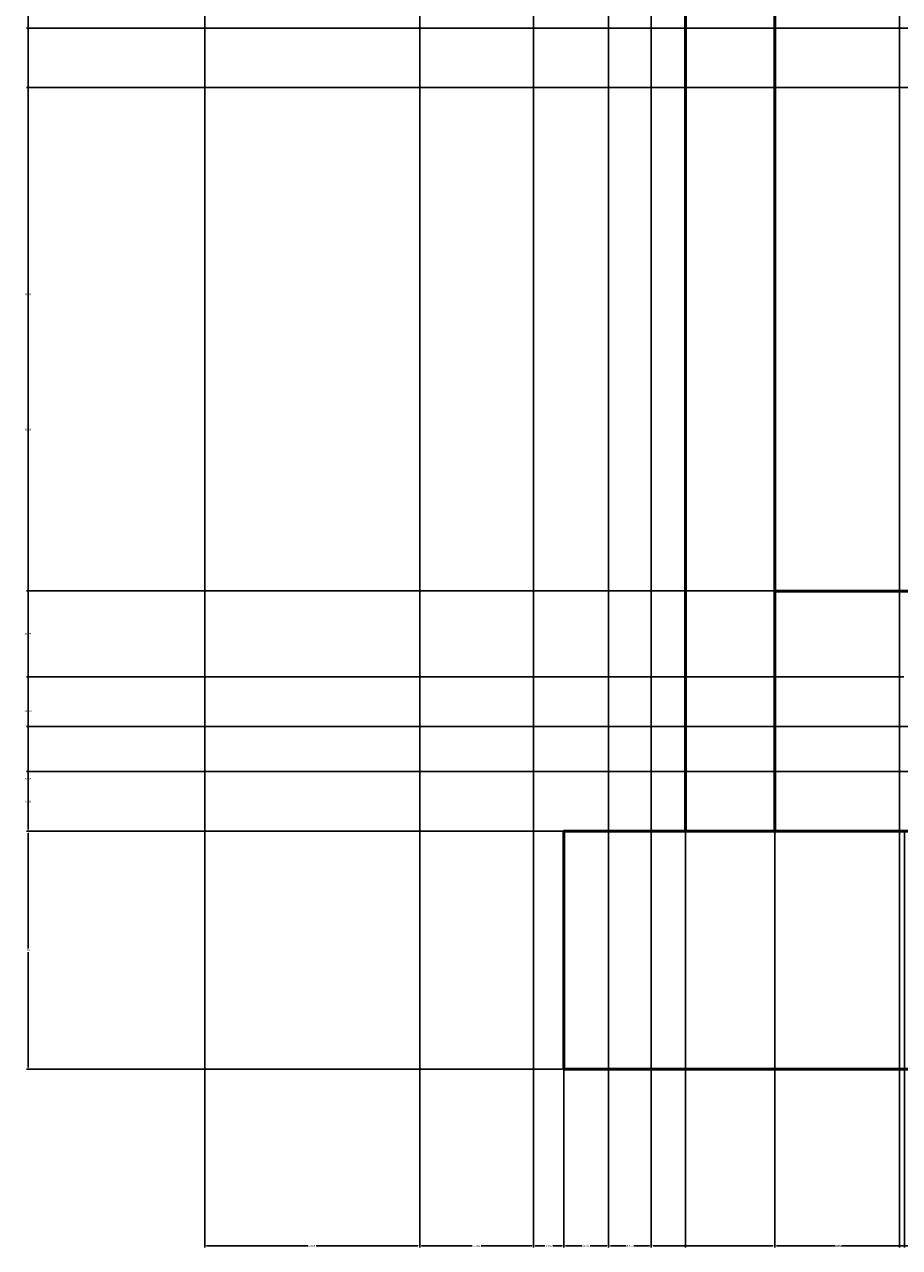
# Model space of a CAD drawing. Units: inches. Extents: x 27 to 409, y -26 to 294.
# Tile 1 of 7: x 27 to 116, y -26 to 97. Entities that reach past the tile are written whole.
import ezdxf

# ---------------------------------------------------------------- set-up
doc = ezdxf.new("R2010")
doc.units = ezdxf.units.IN
doc.header["$MEASUREMENT"] = 0
doc.layers.add('A-ANNO-DIMS', color=2, linetype='Continuous', lineweight=18)
doc.layers.add('A-WALL', color=7, linetype='Continuous', lineweight=50)
doc.styles.get("Standard").update_dxf_attribs({"font": 'arial.ttf'})
doc.dimstyles.get("Standard").update_dxf_attribs({"dimtxt": 0.18, "dimasz": 0.18, "dimexe": 0.18, "dimexo": 0.0625, "dimgap": 0.09, "dimtad": 0, "dimtih": 1, "dimtoh": 1, "dimdec": 4, "dimzin": 0, "dimdsep": 46, "dimtxsty": 'Standard', "dimcen": 0.09, "dimadec": 0, "dimazin": 0, "dimtfac": 1, "dimtdec": 4, "dimtofl": 0, "dimtmove": 0, "dimatfit": 3, "dimfxl": 1, "dimtolj": 1, "dimtzin": 0, "dimarcsym": 0})

# ---------------------------------------------------------------- blocks, each defined once
blk = doc.blocks.new('*D8')
at = {"layer": 'A-ANNO-DIMS', "color": 0, "lineweight": -2, "transparency": 16777216}
for p, q in [((67.27, 209.05), (67.27, -26.5)), ((45.58, 99.43), (45.58, -26.5)), ((45.76, -26.32), (56.03, -26.32)), ((67.09, -26.32), (56.82, -26.32))]:
    blk.add_line(p, q, dxfattribs=at)
at = {"layer": 'A-ANNO-DIMS', "color": 0, "transparency": 16777216}
for points in [[(45.76, -26.29), (45.76, -26.35), (45.58, -26.32)], [(67.09, -26.29), (67.09, -26.35), (67.27, -26.32)]]:
    blk.add_solid(points, dxfattribs=at)
at = {"layer": 'Defpoints', "color": 0, "transparency": 16777216}
for p in [(67.27, 209.11), (45.58, 99.5), (67.27, -26.32)]:
    blk.add_point(p, dxfattribs=at)
at = {"layer": 'A-ANNO-DIMS', "color": 0, "transparency": 16777216, "insert": (56.42, -26.32), "char_height": 0.18, "attachment_point": 5}
blk.add_mtext('\\A1;21.69', dxfattribs=at)
blk = doc.blocks.new('*D9')
at = {"layer": 'A-ANNO-DIMS', "color": 0, "lineweight": -2, "transparency": 16777216}
for p, q in [((78.75, 231.7), (78.75, -26.5)), ((67.27, 209.05), (67.27, -26.5)), ((67.45, -26.32), (72.55, -26.32)), ((78.57, -26.32), (73.46, -26.32))]:
    blk.add_line(p, q, dxfattribs=at)
at = {"layer": 'A-ANNO-DIMS', "color": 0, "transparency": 16777216}
for points in [[(67.45, -26.29), (67.45, -26.35), (67.27, -26.32)], [(78.57, -26.29), (78.57, -26.35), (78.75, -26.32)]]:
    blk.add_solid(points, dxfattribs=at)
at = {"layer": 'Defpoints', "color": 0, "transparency": 16777216}
for p in [(78.75, 231.76), (67.27, 209.11), (78.75, -26.32)]:
    blk.add_point(p, dxfattribs=at)
at = {"layer": 'A-ANNO-DIMS', "color": 0, "transparency": 16777216, "insert": (73.01, -26.32), "char_height": 0.18, "attachment_point": 5}
blk.add_mtext('\\A1;11.482', dxfattribs=at)
blk = doc.blocks.new('*D10')
at = {"layer": 'A-ANNO-DIMS', "color": 0, "lineweight": -2, "transparency": 16777216}
for p, q in [((78.75, 231.7), (78.75, -26.5)), ((81.81, -8.58), (81.81, -26.5)), ((78.93, -26.32), (79.89, -26.32)), ((81.63, -26.32), (80.68, -26.32))]:
    blk.add_line(p, q, dxfattribs=at)
at = {"layer": 'A-ANNO-DIMS', "color": 0, "transparency": 16777216}
for points in [[(78.93, -26.29), (78.93, -26.35), (78.75, -26.32)], [(81.63, -26.29), (81.63, -26.35), (81.81, -26.32)]]:
    blk.add_solid(points, dxfattribs=at)
at = {"layer": 'Defpoints', "color": 0, "transparency": 16777216}
for p in [(78.75, 231.76), (81.81, -8.52), (81.81, -26.32)]:
    blk.add_point(p, dxfattribs=at)
at = {"layer": 'A-ANNO-DIMS', "color": 0, "transparency": 16777216, "insert": (80.28, -26.32), "char_height": 0.18, "attachment_point": 5}
blk.add_mtext('\\A1;3.064', dxfattribs=at)
blk = doc.blocks.new('*D11')
at = {"layer": 'A-ANNO-DIMS', "color": 0, "lineweight": -2, "transparency": 16777216}
for p, q in [((86.32, 163.84), (86.32, -26.5)), ((81.81, -8.58), (81.81, -26.5)), ((81.99, -26.32), (83.67, -26.32)), ((86.14, -26.32), (84.46, -26.32))]:
    blk.add_line(p, q, dxfattribs=at)
at = {"layer": 'A-ANNO-DIMS', "color": 0, "transparency": 16777216}
for points in [[(81.99, -26.29), (81.99, -26.35), (81.81, -26.32)], [(86.14, -26.29), (86.14, -26.35), (86.32, -26.32)]]:
    blk.add_solid(points, dxfattribs=at)
at = {"layer": 'Defpoints', "color": 0, "transparency": 16777216}
for p in [(86.32, 163.9), (81.81, -8.52), (86.32, -26.32)]:
    blk.add_point(p, dxfattribs=at)
at = {"layer": 'A-ANNO-DIMS', "color": 0, "transparency": 16777216, "insert": (84.07, -26.32), "char_height": 0.18, "attachment_point": 5}
blk.add_mtext('\\A1;4.503', dxfattribs=at)
blk = doc.blocks.new('*D12')
at = {"layer": 'A-ANNO-DIMS', "color": 0, "lineweight": -2, "transparency": 16777216}
for p, q in [((90.63, 195.36), (90.63, -26.5)), ((86.32, 163.84), (86.32, -26.5)), ((86.5, -26.32), (88.09, -26.32)), ((90.45, -26.32), (88.85, -26.32))]:
    blk.add_line(p, q, dxfattribs=at)
at = {"layer": 'A-ANNO-DIMS', "color": 0, "transparency": 16777216}
for points in [[(86.5, -26.29), (86.5, -26.35), (86.32, -26.32)], [(90.45, -26.29), (90.45, -26.35), (90.63, -26.32)]]:
    blk.add_solid(points, dxfattribs=at)
at = {"layer": 'Defpoints', "color": 0, "transparency": 16777216}
for p in [(90.63, 195.42), (86.32, 163.9), (90.63, -26.32)]:
    blk.add_point(p, dxfattribs=at)
at = {"layer": 'A-ANNO-DIMS', "color": 0, "transparency": 16777216, "insert": (88.47, -26.32), "char_height": 0.18, "attachment_point": 5}
blk.add_mtext('\\A1;4.311', dxfattribs=at)
blk = doc.blocks.new('*D13')
at = {"layer": 'A-ANNO-DIMS', "color": 0, "lineweight": -2, "transparency": 16777216}
for p, q in [((90.63, 195.36), (90.63, -26.5)), ((103.08, 162.87), (103.08, -26.5)), ((90.81, -26.32), (96.4, -26.32)), ((102.9, -26.32), (97.31, -26.32))]:
    blk.add_line(p, q, dxfattribs=at)
at = {"layer": 'A-ANNO-DIMS', "color": 0, "transparency": 16777216}
for points in [[(90.81, -26.29), (90.81, -26.35), (90.63, -26.32)], [(102.9, -26.29), (102.9, -26.35), (103.08, -26.32)]]:
    blk.add_solid(points, dxfattribs=at)
at = {"layer": 'Defpoints', "color": 0, "transparency": 16777216}
for p in [(90.63, 195.42), (103.08, 162.94), (103.08, -26.32)]:
    blk.add_point(p, dxfattribs=at)
at = {"layer": 'A-ANNO-DIMS', "color": 0, "transparency": 16777216, "insert": (96.85, -26.32), "char_height": 0.18, "attachment_point": 5}
blk.add_mtext('\\A1;12.447', dxfattribs=at)
blk = doc.blocks.new('*D14')
at = {"layer": 'A-ANNO-DIMS', "color": 0, "lineweight": -2, "transparency": 16777216}
for p, q in [((103.08, 162.87), (103.08, -26.5)), ((115.67, 115.93), (115.67, -26.5)), ((103.26, -26.32), (108.93, -26.32)), ((115.49, -26.32), (109.81, -26.32))]:
    blk.add_line(p, q, dxfattribs=at)
at = {"layer": 'A-ANNO-DIMS', "color": 0, "transparency": 16777216}
for points in [[(103.26, -26.29), (103.26, -26.35), (103.08, -26.32)], [(115.49, -26.29), (115.49, -26.35), (115.67, -26.32)]]:
    blk.add_solid(points, dxfattribs=at)
at = {"layer": 'Defpoints', "color": 0, "transparency": 16777216}
for p in [(103.08, 162.94), (115.67, 116), (115.67, -26.32)]:
    blk.add_point(p, dxfattribs=at)
at = {"layer": 'A-ANNO-DIMS', "color": 0, "transparency": 16777216, "insert": (109.37, -26.32), "char_height": 0.18, "attachment_point": 5}
blk.add_mtext('\\A1;12.591', dxfattribs=at)
blk = doc.blocks.new('*D15')
at = {"layer": 'A-ANNO-DIMS', "color": 0, "lineweight": -2, "transparency": 16777216}
for p, q in [((152.83, 275.59), (152.83, -26.5)), ((115.67, 115.93), (115.67, -26.5)), ((115.85, -26.32), (133.86, -26.32)), ((152.65, -26.32), (134.64, -26.32))]:
    blk.add_line(p, q, dxfattribs=at)
at = {"layer": 'A-ANNO-DIMS', "color": 0, "transparency": 16777216}
for points in [[(115.85, -26.29), (115.85, -26.35), (115.67, -26.32)], [(152.65, -26.29), (152.65, -26.35), (152.83, -26.32)]]:
    blk.add_solid(points, dxfattribs=at)
at = {"layer": 'Defpoints', "color": 0, "transparency": 16777216}
for p in [(152.83, 275.65), (115.67, 116), (152.83, -26.32)]:
    blk.add_point(p, dxfattribs=at)
at = {"layer": 'A-ANNO-DIMS', "color": 0, "transparency": 16777216, "insert": (134.25, -26.32), "char_height": 0.18, "attachment_point": 5}
blk.add_mtext('\\A1;37.17', dxfattribs=at)
blk = doc.blocks.new('*D26')
at = {"layer": 'A-ANNO-DIMS', "color": 0, "lineweight": -2, "transparency": 16777216}
for p, q in [((81.75, 15.48), (27.6, 15.48)), ((27.78, 15.3), (27.78, 3.66)), ((27.78, -8.34), (27.78, 3.3)), ((81.75, -8.52), (27.6, -8.52))]:
    blk.add_line(p, q, dxfattribs=at)
at = {"layer": 'A-ANNO-DIMS', "color": 0, "transparency": 16777216}
for points in [[(27.75, 15.3), (27.81, 15.3), (27.78, 15.48)], [(27.75, -8.34), (27.81, -8.34), (27.78, -8.52)]]:
    blk.add_solid(points, dxfattribs=at)
at = {"layer": 'Defpoints', "color": 0, "transparency": 16777216}
for p in [(27.78, 15.48), (81.81, 15.48), (81.81, -8.52)]:
    blk.add_point(p, dxfattribs=at)
at = {"layer": 'A-ANNO-DIMS', "color": 0, "transparency": 16777216, "insert": (27.78, 3.48), "char_height": 0.18, "attachment_point": 5}
blk.add_mtext('\\A1;24', dxfattribs=at)
blk = doc.blocks.new('*D27')
at = {"layer": 'A-ANNO-DIMS', "color": 0, "lineweight": -2, "transparency": 16777216}
for p, q in [((115.6, 39.71), (27.6, 39.71)), ((27.78, 39.53), (27.78, 27.78)), ((27.78, 15.66), (27.78, 27.42)), ((81.75, 15.48), (27.6, 15.48))]:
    blk.add_line(p, q, dxfattribs=at)
at = {"layer": 'A-ANNO-DIMS', "color": 0, "transparency": 16777216}
for points in [[(27.75, 39.53), (27.81, 39.53), (27.78, 39.71)], [(27.75, 15.66), (27.81, 15.66), (27.78, 15.48)]]:
    blk.add_solid(points, dxfattribs=at)
at = {"layer": 'Defpoints', "color": 0, "transparency": 16777216}
for p in [(27.78, 39.71), (115.67, 39.71), (81.81, 15.48)]:
    blk.add_point(p, dxfattribs=at)
at = {"layer": 'A-ANNO-DIMS', "color": 0, "transparency": 16777216, "insert": (27.78, 27.6), "char_height": 0.18, "attachment_point": 5}
blk.add_mtext('\\A1;24.227', dxfattribs=at)
blk = doc.blocks.new('*D28')
at = {"layer": 'A-ANNO-DIMS', "color": 0, "lineweight": -2, "transparency": 16777216}
for p, q in [((45.51, 99.5), (27.6, 99.5)), ((27.78, 99.32), (27.78, 69.78)), ((27.78, 39.89), (27.78, 69.42)), ((115.6, 39.71), (27.6, 39.71))]:
    blk.add_line(p, q, dxfattribs=at)
at = {"layer": 'A-ANNO-DIMS', "color": 0, "transparency": 16777216}
for points in [[(27.75, 99.32), (27.81, 99.32), (27.78, 99.5)], [(27.75, 39.89), (27.81, 39.89), (27.78, 39.71)]]:
    blk.add_solid(points, dxfattribs=at)
at = {"layer": 'Defpoints', "color": 0, "transparency": 16777216}
for p in [(27.78, 99.5), (45.58, 99.5), (115.67, 39.71)]:
    blk.add_point(p, dxfattribs=at)
at = {"layer": 'A-ANNO-DIMS', "color": 0, "transparency": 16777216, "insert": (27.78, 69.6), "char_height": 0.18, "attachment_point": 5}
blk.add_mtext('\\A1;59.79', dxfattribs=at)
blk = doc.blocks.new('*D69')
at = {"layer": 'A-ANNO-DIMS', "color": 0, "lineweight": -2, "transparency": 16777216}
for p, q in [((200.04, 21.5), (27.6, 21.5)), ((27.78, 21.32), (27.78, 18.67)), ((27.78, 15.66), (27.78, 18.31)), ((190.01, 15.48), (27.6, 15.48))]:
    blk.add_line(p, q, dxfattribs=at)
at = {"layer": 'A-ANNO-DIMS', "color": 0, "transparency": 16777216}
for points in [[(27.75, 21.32), (27.81, 21.32), (27.78, 21.5)], [(27.75, 15.66), (27.81, 15.66), (27.78, 15.48)]]:
    blk.add_solid(points, dxfattribs=at)
at = {"layer": 'Defpoints', "color": 0, "transparency": 16777216}
for p in [(27.78, 21.5), (200.1, 21.5), (190.08, 15.48)]:
    blk.add_point(p, dxfattribs=at)
at = {"layer": 'A-ANNO-DIMS', "color": 0, "transparency": 16777216, "insert": (27.78, 18.49), "char_height": 0.18, "attachment_point": 5}
blk.add_mtext('\\A1;6.013', dxfattribs=at)
blk = doc.blocks.new('*D70')
at = {"layer": 'A-ANNO-DIMS', "color": 0, "lineweight": -2, "transparency": 16777216}
for p, q in [((200.04, 90.47), (27.6, 90.47)), ((27.78, 90.29), (27.78, 56.17)), ((27.78, 21.68), (27.78, 55.8)), ((200.04, 21.5), (27.6, 21.5))]:
    blk.add_line(p, q, dxfattribs=at)
at = {"layer": 'A-ANNO-DIMS', "color": 0, "transparency": 16777216}
for points in [[(27.75, 90.29), (27.81, 90.29), (27.78, 90.47)], [(27.75, 21.68), (27.81, 21.68), (27.78, 21.5)]]:
    blk.add_solid(points, dxfattribs=at)
at = {"layer": 'Defpoints', "color": 0, "transparency": 16777216}
for p in [(27.78, 90.47), (200.1, 90.47), (200.1, 21.5)]:
    blk.add_point(p, dxfattribs=at)
at = {"layer": 'A-ANNO-DIMS', "color": 0, "transparency": 16777216, "insert": (27.78, 55.98), "char_height": 0.18, "attachment_point": 5}
blk.add_mtext('\\A1;68.98', dxfattribs=at)
blk = doc.blocks.new('*D71')
at = {"layer": 'A-ANNO-DIMS', "color": 0, "lineweight": -2, "transparency": 16777216}
for p, q in [((196.04, 96.47), (27.6, 96.47)), ((27.78, 96.29), (27.78, 93.65)), ((27.78, 90.65), (27.78, 93.29)), ((200.04, 90.47), (27.6, 90.47))]:
    blk.add_line(p, q, dxfattribs=at)
at = {"layer": 'A-ANNO-DIMS', "color": 0, "transparency": 16777216}
for points in [[(27.75, 96.29), (27.81, 96.29), (27.78, 96.47)], [(27.75, 90.65), (27.81, 90.65), (27.78, 90.47)]]:
    blk.add_solid(points, dxfattribs=at)
at = {"layer": 'Defpoints', "color": 0, "transparency": 16777216}
for p in [(27.78, 96.47), (196.1, 96.47), (200.1, 90.47)]:
    blk.add_point(p, dxfattribs=at)
at = {"layer": 'A-ANNO-DIMS', "color": 0, "transparency": 16777216, "insert": (27.78, 93.47), "char_height": 0.18, "attachment_point": 5}
blk.add_mtext('\\A1;6', dxfattribs=at)
blk = doc.blocks.new('*D72')
at = {"layer": 'A-ANNO-DIMS', "color": 0, "lineweight": -2, "transparency": 16777216}
for p, q in [((190.01, 99.5), (27.6, 99.5)), ((27.78, 99.32), (27.78, 98.17)), ((27.78, 96.65), (27.78, 97.8)), ((196.04, 96.47), (27.6, 96.47))]:
    blk.add_line(p, q, dxfattribs=at)
at = {"layer": 'A-ANNO-DIMS', "color": 0, "transparency": 16777216}
for points in [[(27.75, 99.32), (27.81, 99.32), (27.78, 99.5)], [(27.75, 96.65), (27.81, 96.65), (27.78, 96.47)]]:
    blk.add_solid(points, dxfattribs=at)
at = {"layer": 'Defpoints', "color": 0, "transparency": 16777216}
for p in [(27.78, 99.5), (190.08, 99.5), (196.1, 96.47)]:
    blk.add_point(p, dxfattribs=at)
at = {"layer": 'A-ANNO-DIMS', "color": 0, "transparency": 16777216, "insert": (27.78, 97.98), "char_height": 0.18, "attachment_point": 5}
blk.add_mtext('\\A1;3.023', dxfattribs=at)
blk = doc.blocks.new('*D90')
at = {"layer": 'A-ANNO-DIMS', "color": 0, "lineweight": -2, "transparency": 16777216}
for p, q in [((94.08, 15.42), (94.08, -26.5)), ((103.08, 15.42), (103.08, -26.5)), ((94.26, -26.32), (98.43, -26.32)), ((102.9, -26.32), (98.72, -26.32))]:
    blk.add_line(p, q, dxfattribs=at)
at = {"layer": 'A-ANNO-DIMS', "color": 0, "transparency": 16777216}
for points in [[(94.26, -26.29), (94.26, -26.35), (94.08, -26.32)], [(102.9, -26.29), (102.9, -26.35), (103.08, -26.32)]]:
    blk.add_solid(points, dxfattribs=at)
at = {"layer": 'Defpoints', "color": 0, "transparency": 16777216}
for p in [(94.08, 15.48), (103.08, 15.48), (103.08, -26.32)]:
    blk.add_point(p, dxfattribs=at)
at = {"layer": 'A-ANNO-DIMS', "color": 0, "transparency": 16777216, "insert": (98.58, -26.32), "char_height": 0.18, "attachment_point": 5}
blk.add_mtext('\\A1;9', dxfattribs=at)
blk = doc.blocks.new('*D91')
at = {"layer": 'A-ANNO-DIMS', "color": 0, "lineweight": -2, "transparency": 16777216}
for p, q in [((103.08, 15.42), (103.08, -26.5)), ((116.16, 15.42), (116.16, -26.5)), ((103.26, -26.32), (109.16, -26.32)), ((115.98, -26.32), (110.07, -26.32))]:
    blk.add_line(p, q, dxfattribs=at)
at = {"layer": 'A-ANNO-DIMS', "color": 0, "transparency": 16777216}
for points in [[(103.26, -26.29), (103.26, -26.35), (103.08, -26.32)], [(115.98, -26.29), (115.98, -26.35), (116.16, -26.32)]]:
    blk.add_solid(points, dxfattribs=at)
at = {"layer": 'Defpoints', "color": 0, "transparency": 16777216}
for p in [(103.08, 15.48), (116.16, 15.48), (116.16, -26.32)]:
    blk.add_point(p, dxfattribs=at)
at = {"layer": 'A-ANNO-DIMS', "color": 0, "transparency": 16777216, "insert": (109.62, -26.32), "char_height": 0.18, "attachment_point": 5}
blk.add_mtext('\\A1;13.089', dxfattribs=at)
blk = doc.blocks.new('*D96')
at = {"layer": 'A-ANNO-DIMS', "color": 0, "lineweight": -2, "transparency": 16777216}
for p, q in [((103.08, 39.77), (103.08, 293.63)), ((115.67, 99.56), (115.67, 293.63)), ((103.26, 293.45), (108.93, 293.45)), ((115.49, 293.45), (109.81, 293.45))]:
    blk.add_line(p, q, dxfattribs=at)
at = {"layer": 'A-ANNO-DIMS', "color": 0, "transparency": 16777216}
for points in [[(103.26, 293.48), (103.26, 293.42), (103.08, 293.45)], [(115.49, 293.48), (115.49, 293.42), (115.67, 293.45)]]:
    blk.add_solid(points, dxfattribs=at)
at = {"layer": 'Defpoints', "color": 0, "transparency": 16777216}
for p in [(115.67, 293.45), (115.67, 99.5), (103.08, 39.71)]:
    blk.add_point(p, dxfattribs=at)
at = {"layer": 'A-ANNO-DIMS', "color": 0, "transparency": 16777216, "insert": (109.37, 293.45), "char_height": 0.18, "attachment_point": 5}
blk.add_mtext('\\A1;12.591', dxfattribs=at)
blk = doc.blocks.new('*D105')
at = {"layer": 'A-ANNO-DIMS', "color": 0, "lineweight": -2, "transparency": 16777216}
for p, q in [((121.1, 26.04), (27.6, 26.04)), ((27.78, 25.86), (27.78, 20.94)), ((27.78, 15.66), (27.78, 20.58)), ((103.01, 15.48), (27.6, 15.48))]:
    blk.add_line(p, q, dxfattribs=at)
at = {"layer": 'A-ANNO-DIMS', "color": 0, "transparency": 16777216}
for points in [[(27.75, 25.86), (27.81, 25.86), (27.78, 26.04)], [(27.75, 15.66), (27.81, 15.66), (27.78, 15.48)]]:
    blk.add_solid(points, dxfattribs=at)
at = {"layer": 'Defpoints', "color": 0, "transparency": 16777216}
for p in [(27.78, 26.04), (121.16, 26.04), (103.08, 15.48)]:
    blk.add_point(p, dxfattribs=at)
at = {"layer": 'A-ANNO-DIMS', "color": 0, "transparency": 16777216, "insert": (27.78, 20.76), "char_height": 0.18, "attachment_point": 5}
blk.add_mtext('\\A1;10.56', dxfattribs=at)
blk = doc.blocks.new('*D106')
at = {"layer": 'A-ANNO-DIMS', "color": 0, "lineweight": -2, "transparency": 16777216}
for p, q in [((116.1, 31.04), (27.6, 31.04)), ((27.78, 30.86), (27.78, 28.72)), ((27.78, 26.22), (27.78, 28.36)), ((121.1, 26.04), (27.6, 26.04))]:
    blk.add_line(p, q, dxfattribs=at)
at = {"layer": 'A-ANNO-DIMS', "color": 0, "transparency": 16777216}
for points in [[(27.75, 30.86), (27.81, 30.86), (27.78, 31.04)], [(27.75, 26.22), (27.81, 26.22), (27.78, 26.04)]]:
    blk.add_solid(points, dxfattribs=at)
at = {"layer": 'Defpoints', "color": 0, "transparency": 16777216}
for p in [(27.78, 31.04), (116.16, 31.04), (121.16, 26.04)]:
    blk.add_point(p, dxfattribs=at)
at = {"layer": 'A-ANNO-DIMS', "color": 0, "transparency": 16777216, "insert": (27.78, 28.54), "char_height": 0.18, "attachment_point": 5}
blk.add_mtext('\\A1;5', dxfattribs=at)
blk = doc.blocks.new('*D107')
at = {"layer": 'A-ANNO-DIMS', "color": 0, "lineweight": -2, "transparency": 16777216}
for p, q in [((103.01, 39.71), (27.6, 39.71)), ((27.78, 39.53), (27.78, 35.56)), ((27.78, 31.22), (27.78, 35.19)), ((116.1, 31.04), (27.6, 31.04))]:
    blk.add_line(p, q, dxfattribs=at)
at = {"layer": 'A-ANNO-DIMS', "color": 0, "transparency": 16777216}
for points in [[(27.75, 39.53), (27.81, 39.53), (27.78, 39.71)], [(27.75, 31.22), (27.81, 31.22), (27.78, 31.04)]]:
    blk.add_solid(points, dxfattribs=at)
at = {"layer": 'Defpoints', "color": 0, "transparency": 16777216}
for p in [(27.78, 39.71), (103.08, 39.71), (116.16, 31.04)]:
    blk.add_point(p, dxfattribs=at)
at = {"layer": 'A-ANNO-DIMS', "color": 0, "transparency": 16777216, "insert": (27.78, 35.38), "char_height": 0.18, "attachment_point": 5}
blk.add_mtext('\\A1;8.666', dxfattribs=at)

msp = doc.modelspace()

# ---------------------------------------------------------------- linework, layer by layer
at = {"layer": 'A-WALL'}
for p, q in [((94.0751, 99.4952), (94.0751, 15.4825)), ((103.0751, 99.4952), (103.0751, 15.4825)), ((103.0751, 39.7093), (166.0751, 39.7093)), ((94.0751, 15.4825), (334.0751, 15.4825))]:
    msp.add_line(p, q, dxfattribs=at)
msp.add_lwpolyline([(187.493, 15.4825), (81.814, 15.4825), (81.814, -8.5175), (187.493, -8.5175)], close=True, dxfattribs=at)

# ---------------------------------------------------------------- dimensions: what is measured, and where the dimension line sits
at = {"layer": 'A-ANNO-DIMS'}
for base, p1, p2, override, picture, middle in [((115.66655, 293.45166), (103.07506, 39.70931), (115.66655, 99.49521), {"dimdec": 3, "dimlfac": 1, "dimrnd": 0, "dimzin": 0, "dimdsep": 46, "dimlunit": 2}, '*D96', (109.3708, 293.45166)), ((152.833, -26.3175), (115.6666, 115.9951), (152.833, 275.6517), {"dimdec": 2, "dimlfac": 1, "dimrnd": 0, "dimzin": 0, "dimdsep": 46, "dimlunit": 2}, '*D15', (134.2498, -26.3175)), ((78.7499, -26.3175), (67.2675, 209.1141), (78.7499, 231.7582), {"dimdec": 3, "dimlfac": 1, "dimrnd": 0, "dimzin": 0, "dimdsep": 46, "dimlunit": 2}, '*D9', (73.0087, -26.3175)), ((81.814, -26.3175), (78.7499, 231.7582), (81.814, -8.5175), {"dimdec": 3, "dimlfac": 1, "dimrnd": 0, "dimzin": 0, "dimdsep": 46, "dimlunit": 2}, '*D10', (80.2819, -26.3175)), ((67.2675, -26.3175), (45.5772, 99.4952), (67.2675, 209.1141), {"dimdec": 2, "dimlfac": 1, "dimrnd": 0, "dimzin": 0, "dimdsep": 46, "dimlunit": 2}, '*D8', (56.4224, -26.3175)), ((90.6277, -26.3175), (86.3168, 163.9028), (90.6277, 195.4248), {"dimdec": 3, "dimlfac": 1, "dimrnd": 0, "dimzin": 0, "dimdsep": 46, "dimlunit": 2}, '*D12', (88.4723, -26.3175)), ((103.0751, -26.3175), (90.6277, 195.4248), (103.0751, 162.937), {"dimdec": 3, "dimlfac": 1, "dimrnd": 0, "dimzin": 0, "dimdsep": 46, "dimlunit": 2}, '*D13', (96.8514, -26.3175)), ((86.3168, -26.3175), (81.814, -8.5175), (86.3168, 163.9028), {"dimdec": 3, "dimlfac": 1, "dimrnd": 0, "dimzin": 0, "dimdsep": 46, "dimlunit": 2}, '*D11', (84.0654, -26.3175)), ((115.66655, -26.31755), (103.07506, 162.93703), (115.66655, 115.99512), {"dimdec": 3, "dimlfac": 1, "dimrnd": 0, "dimzin": 0, "dimdsep": 46, "dimlunit": 2}, '*D14', (109.3708, -26.31755)), ((103.0751, -26.3175), (94.0751, 15.4825), (103.0751, 15.4825), {"dimdec": 0, "dimlfac": 1, "dimrnd": 0, "dimzin": 0, "dimdsep": 46, "dimlunit": 2}, '*D90', (98.5751, -26.3175)), ((116.1637, -26.3175), (103.0751, 15.4825), (116.1637, 15.4825), {"dimdec": 3, "dimlfac": 1, "dimrnd": 0, "dimzin": 0, "dimdsep": 46, "dimlunit": 2}, '*D91', (109.6194, -26.3175))]:
    dim = msp.add_linear_dim(base=base, p1=p1, p2=p2, dimstyle='Standard', override=override, dxfattribs=at)
    dim.commit()
    dim.dimension.update_dxf_attribs({"geometry": picture, "text_midpoint": middle})
for base, p1, p2, override, picture, middle in [((27.7772, 99.4952), (115.6666, 39.7093), (45.5772, 99.4952), {"dimdec": 2, "dimlfac": 1, "dimrnd": 0, "dimzin": 0, "dimdsep": 46, "dimlunit": 2}, '*D28', (27.7772, 69.6023)), ((27.7772, 99.4952), (196.1036, 96.4722), (190.0751, 99.4952), {"dimdec": 3, "dimlfac": 1, "dimrnd": 0, "dimzin": 0, "dimdsep": 46, "dimlunit": 2}, '*D72', (27.7772, 97.9837)), ((27.7772, 96.4722), (200.1036, 90.4722), (196.1036, 96.4722), {"dimdec": 0, "dimlfac": 1, "dimrnd": 0, "dimzin": 0, "dimdsep": 46, "dimlunit": 2}, '*D71', (27.7772, 93.4722)), ((27.7772, 90.4722), (200.1036, 21.4952), (200.1036, 90.4722), {"dimdec": 2, "dimlfac": 1, "dimrnd": 0, "dimzin": 0, "dimdsep": 46, "dimlunit": 2}, '*D70', (27.7772, 55.9837)), ((27.7772, 39.7093), (81.814, 15.4825), (115.6666, 39.7093), {"dimdec": 3, "dimlfac": 1, "dimrnd": 0, "dimzin": 0, "dimdsep": 46, "dimlunit": 2}, '*D27', (27.7772, 27.5959)), ((27.7772, 39.7093), (116.1637, 31.043), (103.0751, 39.7093), {"dimdec": 3, "dimlfac": 1, "dimrnd": 0, "dimzin": 0, "dimdsep": 46, "dimlunit": 2}, '*D107', (27.7772, 35.3761)), ((27.7772, 31.043), (121.1637, 26.043), (116.1637, 31.043), {"dimdec": 0, "dimlfac": 1, "dimrnd": 0, "dimzin": 0, "dimdsep": 46, "dimlunit": 2}, '*D106', (27.7772, 28.543)), ((27.7772, 26.043), (103.0751, 15.4825), (121.1637, 26.043), {"dimdec": 2, "dimlfac": 1, "dimrnd": 0, "dimzin": 0, "dimdsep": 46, "dimlunit": 2}, '*D105', (27.7772, 20.7627)), ((27.7772, 21.4952), (190.0751, 15.4825), (200.1036, 21.4952), {"dimdec": 3, "dimlfac": 1, "dimrnd": 0, "dimzin": 0, "dimdsep": 46, "dimlunit": 2}, '*D69', (27.7772, 18.4888)), ((27.7772, 15.4825), (81.814, -8.5175), (81.814, 15.4825), {"dimdec": 0, "dimlfac": 1, "dimrnd": 0, "dimzin": 0, "dimdsep": 46, "dimlunit": 2}, '*D26', (27.7772, 3.4825))]:
    dim = msp.add_linear_dim(base=base, p1=p1, p2=p2, angle=90, dimstyle='Standard', override=override, dxfattribs=at)
    dim.commit()
    dim.dimension.update_dxf_attribs({"geometry": picture, "text_midpoint": middle})

doc.saveas('drawing.dxf')
